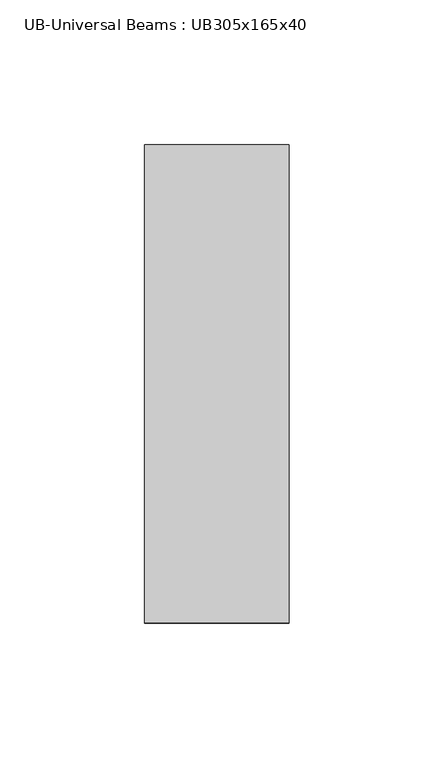
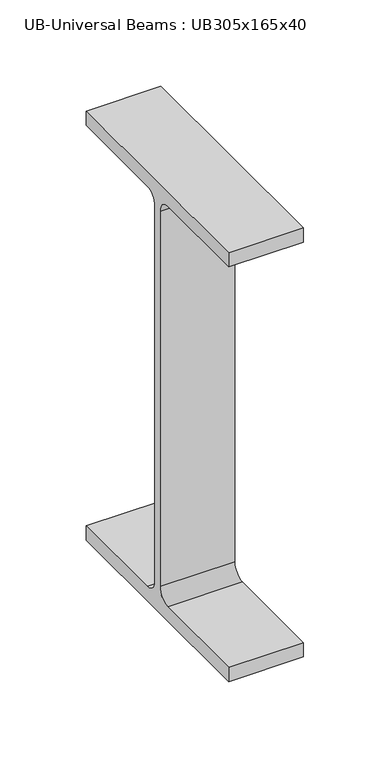
"""IFC4 building model written with IfcOpenShell, lengths in millimetres: beam geometry, UB-Universal Beams : UB305x165x40."""

from ifc_helpers import new_model, si_unit, point, frame, frame_2d, origin, place, context, project, spatial, polyline, circle_curve, trimmed, segment, composite_curve, outline, extrude, source, transform, mapped, element, save


def ub_universal_beams_ub305x165x40_0af343aa(model_context):
    return source(origin(), model_context, "Body", "SweptSolid", [
        extrude(outline(composite_curve([segment(polyline([(82.5, -141.5), (82.5, -151.7), (-82.5, -151.7), (-82.5, -141.5), (-11.9, -141.5)]), True, "CONTINUOUS"), segment(trimmed(circle_curve(frame_2d((-11.9, -132.6)), 8.9), [point((-11.9, -141.5))], [point((-3.0, -132.6))], True, "CARTESIAN"), True, "CONTINUOUS"), segment(polyline([(-3.0, -132.6), (-3.0, 132.6)]), True, "CONTINUOUS"), segment(trimmed(circle_curve(frame_2d((-11.9, 132.6)), 8.9), [point((-3.0, 132.6))], [point((-11.9, 141.5))], True, "CARTESIAN"), True, "CONTINUOUS"), segment(polyline([(-11.9, 141.5), (-82.5, 141.5), (-82.5, 151.7), (82.5, 151.7), (82.5, 141.5), (11.9, 141.5)]), True, "CONTINUOUS"), segment(trimmed(circle_curve(frame_2d((11.9, 132.6)), 8.9), [point((11.9, 141.5))], [point((3.0, 132.6))], True, "CARTESIAN"), True, "CONTINUOUS"), segment(polyline([(3.0, 132.6), (3.0, -132.6)]), True, "CONTINUOUS"), segment(trimmed(circle_curve(frame_2d((11.9, -132.6)), 8.9), [point((3.0, -132.6))], [point((11.9, -141.5))], True, "CARTESIAN"), True, "CONTINUOUS"), segment(polyline([(11.9, -141.5), (82.5, -141.5)]), True, "CONTINUOUS")], self_intersect=False)), frame((-35.6, 0.0, 0.0), z_axis=(1.0, 0.0, 0.0), x_axis=(0.0, 1.0, 0.0)), (0.0, 0.0, 1.0), 49.9),
    ])


if __name__ == "__main__":
    model = new_model("IFC4")
    model_context = context("Model", 3, world=origin())
    ifc_project = project(units=[si_unit("LENGTHUNIT", "METRE", prefix="MILLI")], contexts=[model_context])
    site = spatial("IfcSite", under=ifc_project)
    building = spatial("IfcBuilding", under=site)
    placement = place(None, origin())
    ub_universal_beams_ub305x165x40_shape = ub_universal_beams_ub305x165x40_0af343aa(model_context)
    element("IfcBeam", 1, ObjectType="UB-Universal Beams : UB305x165x40", at=placement, inside=building, context=model_context, shape_type="MappedRepresentation", body=[
        mapped(ub_universal_beams_ub305x165x40_shape, transform((0.0, 0.0, 0.0), x_axis=(1.0, 0.0, 0.0), y_axis=(0.0, 1.0, 0.0), z_axis=(0.0, 0.0, 1.0))),
    ])
    save(model, "model.ifc")

# Revit data of these elements
# Type "UB-Universal Beams : UB305x165x40"
#   Section Name Key = "UB305X165X40"
#   Width = 16.5 cm
#   Web Thickness = 0.6 cm
#   Web Fillet = 0.89 cm
#   Warping Constant = 164000.0 cm⁶
#   Torsional Moment of Inertia = 14.70 cm⁴
#   Section Area = 51.3 cm²
#   Plastic Modulus weak axis = 142.0 cm³
#   Plastic Modulus strong axis = 623.0 cm³
#   Nominal Weight = 40.2999 kgf/m
#   Moment of Inertia weak axis = 764.00 cm⁴
#   Moment of Inertia strong axis = 8503.00 cm⁴
#   Height = 30.34 cm
#   Flange Thickness = 1.02 cm
#   Elastic Modulus weak axis = 92.6 cm³
#   Elastic Modulus strong axis = 560.0 cm³
#   Centroid Vertical = 15.17 cm
#   Centroid Horizontal = 8.25 cm
#   Bolt Spacing = 9.0 cm
#   Length [instance default] = 1500 mm
#   Structural Material [instance default] = Metal - Steel 43-275
#   Type Comments = ""
#   Assembly Code = ""
# Element 1 (IfcBeam, "UB-Universal Beams : UB305x165x40")
#   Materials on its faces: "Metal - Steel 43-275"
# Materials
#   "Metal - Steel 43-275": class "Metal", colour RGB 247 247 247, transparency 0, Cost = 0
